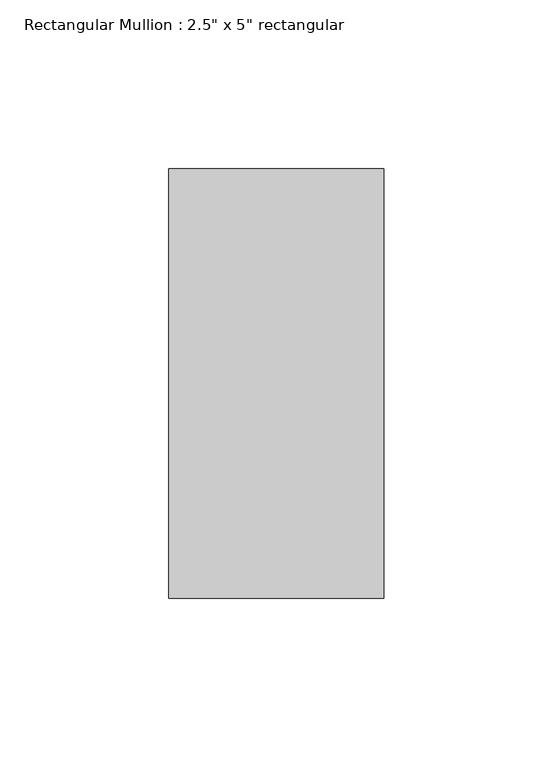
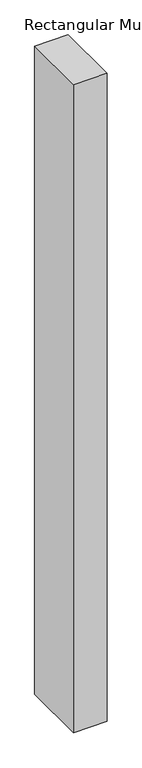
"""IFC4 building model written with IfcOpenShell, lengths in millimetres: member geometry."""

from ifc_helpers import new_model, si_unit, frame, origin, place, context, project, spatial, polyline, outline, extrude, source, transform, mapped, element, save


def member_6146d365(model_context):
    return source(origin(), model_context, "Body", "SweptSolid", [
        extrude(outline(polyline([(0.0, 63.5), (0.0, -63.5), (-63.5, -63.5), (-63.5, 63.5), (0.0, 63.5)])), frame((0.0, 0.0, -1296.7619602), z_axis=(0.0, 0.0, 1.0), x_axis=(1.0, 0.0, 0.0)), (0.0, 0.0, 1.0), 1296.7619602),
    ])


if __name__ == "__main__":
    model = new_model("IFC4")
    model_context = context("Model", 3, world=origin())
    ifc_project = project(units=[si_unit("LENGTHUNIT", "METRE", prefix="MILLI")], contexts=[model_context])
    site = spatial("IfcSite", under=ifc_project)
    building = spatial("IfcBuilding", under=site)
    placement = place(None, origin())
    member_shape = member_6146d365(model_context)
    element("IfcMember", 1, ObjectType="Rectangular Mullion : 2.5\" x 5\" rectangular", at=placement, inside=building, context=model_context, shape_type="MappedRepresentation", body=[
        mapped(member_shape, transform((0.0, 0.0, 0.0), x_axis=(1.0, 0.0, 0.0), y_axis=(0.0, 1.0, 0.0), z_axis=(0.0, 0.0, 1.0))),
    ])
    save(model, "model.ifc")

# Revit data of these elements
# Type "Rectangular Mullion : 2.5\" x 5\" rectangular"
#   built-in parameter 1007304 = 0.416667 (stored number, unit not read)
#   built-in parameter 1007301 = 0.104167 (stored number, unit not read)
#   built-in parameter 1007300 = 0.104167 (stored number, unit not read)
# Element 1 (IfcMember, "Rectangular Mullion : 2.5\" x 5\" rectangular")
#   Materials on its faces: "Aluminum"
# Materials
#   "Aluminum": class "Metal", colour RGB 247 247 247, transparency 0, Description = "Aluminum 6061", Cost = 0
